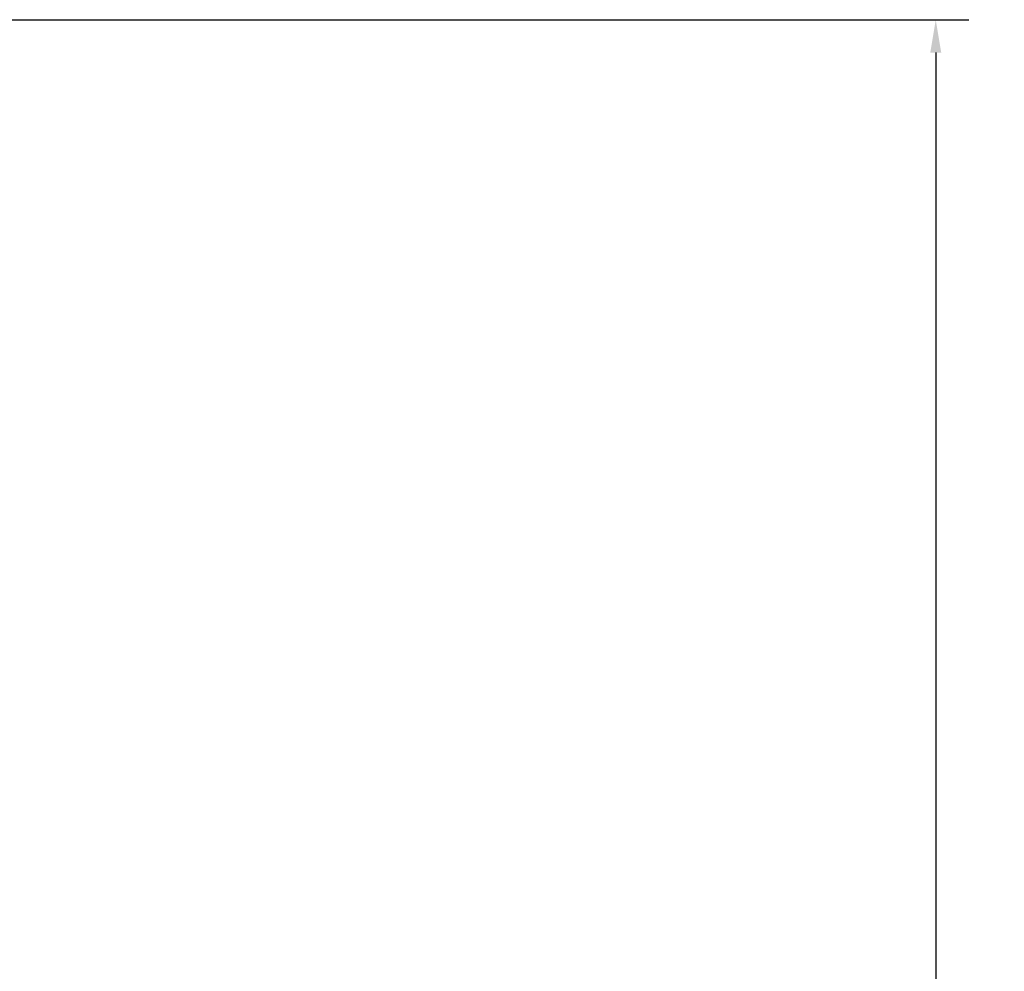
# Model space of a CAD drawing. Units: metres. Extents: x 2031 to 2061.8, y 1886.4 to 1909.8.
# Tile 10 of 10: x 2056.4 to 2061.8, y 1901.9 to 1907.1. Entities that reach past the tile are written whole.
import ezdxf

# ---------------------------------------------------------------- set-up
doc = ezdxf.new("R2010")
doc.units = ezdxf.units.M
doc.layers.add('A-ANNO-DIMS', color=2, linetype='Continuous', lineweight=18)
doc.styles.get("Standard").update_dxf_attribs({"font": 'arial.ttf'})
doc.dimstyles.get("Standard").update_dxf_attribs({"dimtxt": 0.18, "dimasz": 0.18, "dimexe": 0.18, "dimexo": 0.0625, "dimgap": 0.09, "dimtad": 0, "dimtih": 1, "dimtoh": 1, "dimdec": 4, "dimzin": 0, "dimdsep": 46, "dimtxsty": 'Standard', "dimcen": 0.09, "dimadec": 0, "dimazin": 0, "dimtfac": 1, "dimtdec": 4, "dimtofl": 0, "dimtmove": 0, "dimatfit": 3, "dimfxl": 1, "dimtolj": 1, "dimtzin": 0, "dimarcsym": 0})

# ---------------------------------------------------------------- blocks, each defined once
blk = doc.blocks.new('*D45')
at = {"layer": 'A-ANNO-DIMS', "color": 0, "lineweight": -2, "transparency": 16777216}
for p, q in [((2047.556386000001, 1907.081203000001), (2061.614374000002, 1907.081203000001)), ((2061.434374000002, 1906.901203000001), (2061.434374000002, 1897.862029637791)), ((2061.434374000002, 1888.459050000001), (2061.434374000002, 1897.498223362211)), ((2054.286386000001, 1888.279050000001), (2061.614374000002, 1888.279050000001))]:
    blk.add_line(p, q, dxfattribs=at)
at = {"layer": 'A-ANNO-DIMS', "color": 0, "transparency": 16777216}
for points in [[(2061.404374000002, 1906.901203000001), (2061.464374000002, 1906.901203000001), (2061.434374000002, 1907.081203000001)], [(2061.404374000002, 1888.459050000001), (2061.464374000002, 1888.459050000001), (2061.434374000002, 1888.279050000001)]]:
    blk.add_solid(points, dxfattribs=at)
at = {"layer": 'Defpoints', "color": 0, "transparency": 16777216}
for p in [(2047.493886000001, 1907.081203000001), (2061.434374000002, 1907.081203000001), (2054.223886000001, 1888.279050000001)]:
    blk.add_point(p, dxfattribs=at)
at = {"layer": 'A-ANNO-DIMS', "color": 0, "transparency": 16777216, "insert": (2061.434374000002, 1897.6801265), "char_height": 0.18, "attachment_point": 5}
blk.add_mtext('\\A1;18.802', dxfattribs=at)

msp = doc.modelspace()

# ---------------------------------------------------------------- dimensions: what is measured, and where the dimension line sits
at = {"layer": 'A-ANNO-DIMS'}
dim = msp.add_linear_dim(base=(2061.434374000002, 1907.081203000001), p1=(2054.223886, 1888.27905), p2=(2047.493886, 1907.081203), angle=90, dimstyle='Standard', override={"dimdec": 3, "dimlfac": 1, "dimrnd": 0, "dimzin": 0, "dimdsep": 46, "dimlunit": 2}, dxfattribs=at)
dim.commit()
dim.dimension.update_dxf_attribs({"geometry": '*D45', "text_midpoint": (2061.434374000002, 1897.6801265)})

doc.saveas('drawing.dxf')
